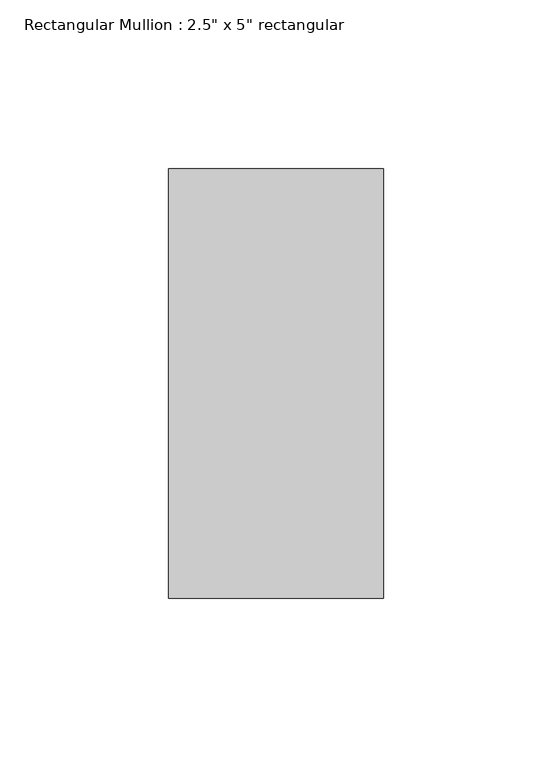
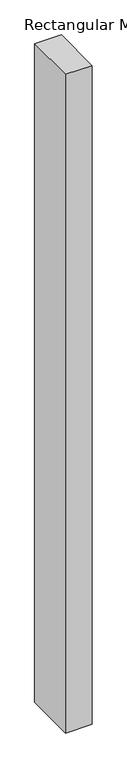
"""IFC4 building model written with IfcOpenShell, lengths in millimetres: member geometry."""

from ifc_helpers import new_model, si_unit, frame, origin, place, context, project, spatial, polyline, outline, extrude, source, transform, mapped, element, save


def member_224a2a57(model_context):
    return source(origin(), model_context, "Body", "SweptSolid", [
        extrude(outline(polyline([(0.0, 63.5), (0.0, -63.5), (-63.5, -63.5), (-63.5, 63.5), (0.0, 63.5)])), frame((0.0, 0.0, -1656.4112238), z_axis=(0.0, 0.0, 1.0), x_axis=(1.0, 0.0, 0.0)), (0.0, 0.0, 1.0), 1656.4112238),
    ])


if __name__ == "__main__":
    model = new_model("IFC4")
    model_context = context("Model", 3, world=origin())
    ifc_project = project(units=[si_unit("LENGTHUNIT", "METRE", prefix="MILLI")], contexts=[model_context])
    site = spatial("IfcSite", under=ifc_project)
    building = spatial("IfcBuilding", under=site)
    placement = place(None, origin())
    member_shape = member_224a2a57(model_context)
    element("IfcMember", 1, ObjectType="Rectangular Mullion : 2.5\" x 5\" rectangular", at=placement, inside=building, context=model_context, shape_type="MappedRepresentation", body=[
        mapped(member_shape, transform((0.0, 0.0, 0.0), x_axis=(1.0, 0.0, 0.0), y_axis=(0.0, 1.0, 0.0), z_axis=(0.0, 0.0, 1.0))),
    ])
    save(model, "model.ifc")

# Revit data of these elements
# Type "Rectangular Mullion : 2.5\" x 5\" rectangular"
#   built-in parameter 1007304 = 0.416667 (stored number, unit not read)
#   built-in parameter 1007301 = 0.104167 (stored number, unit not read)
#   built-in parameter 1007300 = 0.104167 (stored number, unit not read)
# Element 1 (IfcMember, "Rectangular Mullion : 2.5\" x 5\" rectangular")
#   Materials on its faces: "Aluminum"
# Materials
#   "Aluminum": class "Metal", colour RGB 247 247 247, transparency 0, Description = "Aluminum 6061", Cost = 0
